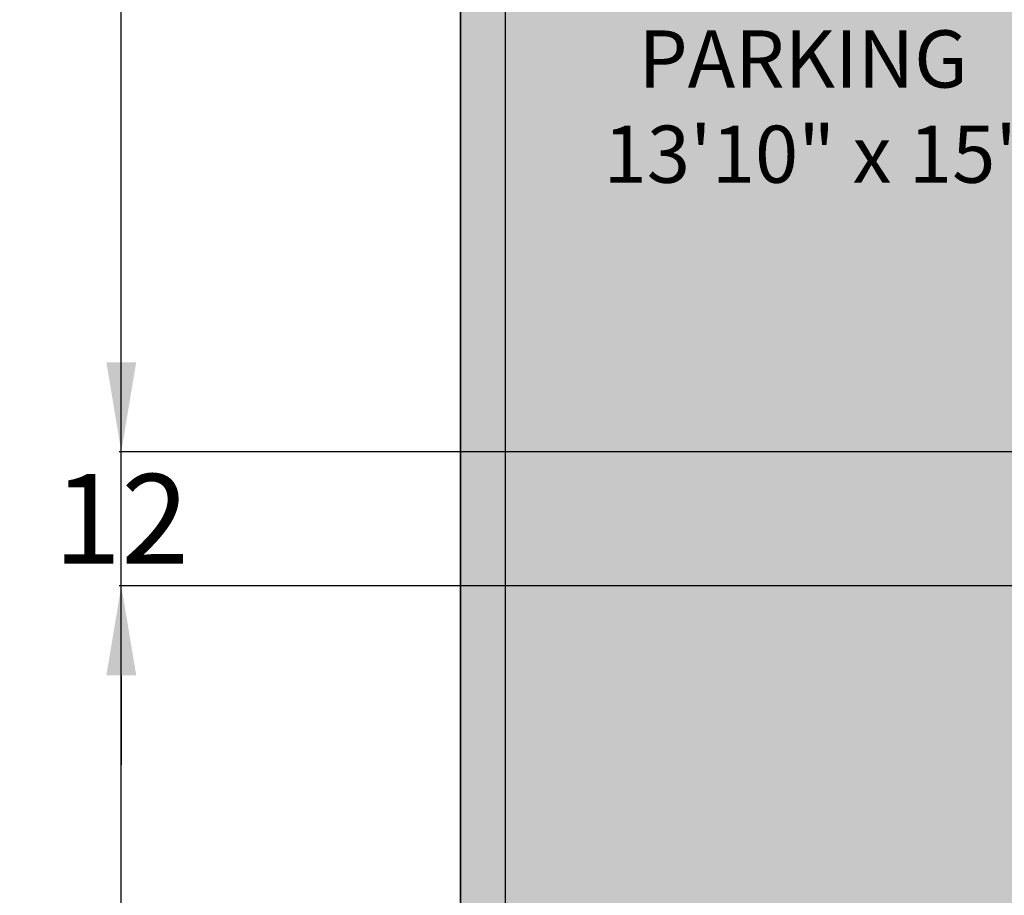
# Model space of a CAD drawing. Units: inches. Extents: x 389 to 971, y 148 to 870.
# Tile 2 of 14: x 389 to 477, y 349 to 428. Entities that reach past the tile are written whole.
import ezdxf

# ---------------------------------------------------------------- set-up
doc = ezdxf.new("R2010")
doc.units = ezdxf.units.IN
doc.header["$MEASUREMENT"] = 0
for name, color, linetype, lineweight in [('A-ANNO-DIMS', 2, 'Continuous', 18), ('A-AREA-IDEN', 7, 'Continuous', 18), ('C-PROP', 7, 'Continuous', 35), ('L-GRND-BASE-PATT', 8, 'Continuous', 13), ('L-WALL', 7, 'Continuous', 30)]:
    doc.layers.add(name, color=color, linetype=linetype, lineweight=lineweight)
doc.layers.add('A-WALL-PATT', color=18, linetype='Continuous', lineweight=13, true_color=0x000000)
doc.layers.add('L-GRND-PATT', color=39, linetype='Continuous', lineweight=13, true_color=0x603913)
doc.styles.get("Standard").update_dxf_attribs({"font": 'arial.ttf'})
doc.dimstyles.get("Standard").update_dxf_attribs({"dimtxt": 8, "dimasz": 8, "dimexe": 0.18, "dimexo": 0.0625, "dimgap": 0.09, "dimtad": 0, "dimtih": 1, "dimtoh": 1, "dimdec": 0, "dimzin": 0, "dimdsep": 46, "dimlunit": 3, "dimtxsty": 'Standard', "dimcen": 0.09, "dimadec": 0, "dimazin": 0, "dimtfac": 1, "dimtdec": 0, "dimtofl": 0, "dimtmove": 0, "dimatfit": 3, "dimfxl": 1, "dimtolj": 1, "dimtzin": 0, "dimarcsym": 0})

# ---------------------------------------------------------------- blocks, each defined once
blk = doc.blocks.new('*D45')
at = {"layer": 'A-ANNO-DIMS', "color": 0, "lineweight": -2, "transparency": 16777216}
for p, q in [((428.1535240000002, 834.6445130000004), (397.7110240000004, 834.6445130000004)), ((397.8910240000004, 826.6445130000004), (397.8910240000005, 538.8190969017736)), ((397.8910240000005, 242.6445130000001), (397.8910240000005, 530.4699290982267)), ((428.1535240000002, 234.6445130000001), (397.7110240000005, 234.6445130000001))]:
    blk.add_line(p, q, dxfattribs=at)
at = {"layer": 'A-ANNO-DIMS', "color": 0, "transparency": 16777216}
for points in [[(396.5576906666671, 826.6445130000004), (399.2243573333337, 826.6445130000004), (397.8910240000004, 834.6445130000004)], [(396.5576906666672, 242.6445130000001), (399.2243573333338, 242.6445130000001), (397.8910240000005, 234.6445130000001)]]:
    blk.add_solid(points, dxfattribs=at)
at = {"layer": 'Defpoints', "color": 0, "transparency": 16777216}
for p in [(397.8910240000004, 834.6445130000004), (428.2160240000002, 834.6445130000004), (428.2160240000002, 234.6445130000001)]:
    blk.add_point(p, dxfattribs=at)
at = {"layer": 'A-ANNO-DIMS', "color": 0, "transparency": 16777216, "insert": (397.8910240000005, 534.6445129999998), "char_height": 8, "attachment_point": 5}
blk.add_mtext('\\A1;600', dxfattribs=at)
blk = doc.blocks.new('*D53')
at = {"layer": 'A-ANNO-DIMS', "color": 0, "lineweight": -2, "transparency": 16777216}
for p, q in [((397.8910240000004, 396.9189020000002), (397.8910240000004, 404.9189020000001)), ((690.1535240000002, 388.9189020000003), (397.7110240000004, 388.9189020000002)), ((690.1535240000002, 376.9189020000001), (397.7110240000005, 376.9189020000001)), ((397.8910240000005, 368.9189020000001), (397.8910240000005, 360.918902))]:
    blk.add_line(p, q, dxfattribs=at)
at = {"layer": 'A-ANNO-DIMS', "color": 0, "transparency": 16777216}
for points in [[(396.5576906666671, 396.9189020000002), (399.2243573333337, 396.9189020000002), (397.8910240000004, 388.9189020000002)], [(396.5576906666671, 368.9189020000001), (399.2243573333338, 368.9189020000001), (397.8910240000005, 376.9189020000001)]]:
    blk.add_solid(points, dxfattribs=at)
at = {"layer": 'Defpoints', "color": 0, "transparency": 16777216}
for p in [(397.8910240000004, 388.9189020000002), (690.2160240000001, 388.9189020000003), (690.2160240000001, 376.9189020000001)]:
    blk.add_point(p, dxfattribs=at)
at = {"layer": 'A-ANNO-DIMS', "color": 0, "transparency": 16777216, "insert": (397.8910240000004, 382.9189019999999), "char_height": 8, "attachment_point": 5}
blk.add_mtext('\\A1;12', dxfattribs=at)

msp = doc.modelspace()

# ---------------------------------------------------------------- hatches: boundary and pattern name
at = {"layer": 'A-WALL-PATT'}
h = msp.add_hatch(color=256, dxfattribs=at)
h.dxf.hatch_style = 1
h.paths.add_polyline_path([(432.2160244416713, 434.6445131961097), (436.3672936601142, 434.6445131961097), (436.3672936601142, 443.6445131961098), (432.2160244416713, 443.6445131961098), (432.2160244416714, 830.6445131961094), (746.2160244416714, 830.6445131961098), (746.2160244416714, 823.8175070811654), (755.2160244416712, 823.8175070811657), (755.2160244416712, 825.6445131961098), (839.2160244416713, 825.6445131961098), (839.2160244416713, 803.5176064986067), (839.2160244416712, 741.6445131961098), (755.2160244416712, 741.6445131961098), (755.2160244416712, 748.4596256139029), (755.1858732057922, 748.4596256139029), (750.7160244416712, 748.4596256139029), (746.2160244416714, 748.4596256139029), (746.2160244416714, 732.6445131961098), (839.2160244416712, 732.6445131961098), (839.2160244416712, 600.6445131961098), (708.5170970640701, 600.6445131961098), (708.5170970640701, 596.1445131961098), (708.5170970640701, 591.6445131961098), (794.2160244416712, 591.6445131961098), (794.2160244416712, 587.4291281246713), (803.2160244416712, 587.4291281246713), (803.2160244416712, 591.6445131961098), (839.2160244416712, 591.6445131961098), (839.2160244416712, 466.6011988194286), (803.2160244416712, 466.6011988194285), (803.2160244416712, 471.0308934694551), (794.2160244416712, 471.0308934694551), (794.2160244416712, 466.6011988194285), (784.6144969105871, 466.6011988194285), (784.6144969105871, 457.6011988194286), (839.2160244416712, 457.6011988194286), (839.2160244416712, 447.6445131961096), (839.2160244416713, 294.6445131961098), (810.0513609197294, 294.6445131961098), (810.0513609197296, 285.6445131961097), (839.2160244416713, 285.6445131961097), (839.2160244416713, 238.6445131961098), (590.2160244416713, 238.6445131961097), (590.2160244416713, 234.6445131961098), (848.2160244416714, 234.6445131961098), (848.2160244416714, 834.6445131961098), (428.2160244416714, 834.6445131961098), (428.2160244416714, 234.6445131961098), (437.2160244416714, 234.6445131961098), (437.2160244416714, 243.6445131961098), (432.2160244416713, 243.6445131961098)])
at = {"layer": 'L-GRND-BASE-PATT'}
h = msp.add_hatch(color=256, dxfattribs=at)
h.dxf.hatch_style = 1
edge = h.paths.add_edge_path(flags=16)
edge.add_ellipse((8782.002602781105, 354.2472542798386), major_axis=(-8296.949265805946, 5.39345e-11), ratio=0.8423038695428886, start_angle=-0.0902290885933894, end_angle=0.3838667787920258, ccw=False)
edge.add_ellipse((485.0533369751568, 368.2895347624687), major_axis=(-1.159084047334488, 1.838e-13), ratio=0.8423038695439892, start_angle=9.094947017729282e-12, end_angle=90.00000000000898, ccw=False)
edge.add_line((483.8942529278224, 368.2895347624687), (483.8942529278225, 387.6039063360424))
edge.add_ellipse((485.0533369751571, 387.2465553762829), major_axis=(1.159084047334488, 1.838e-13), ratio=0.8423038695439892, start_angle=89.99999999999102, end_angle=179.9999999999909, ccw=False)
edge.add_line((485.0533369751572, 388.2228563544795), (485.5047440247956, 388.2228563544795))
edge.add_ellipse((898.8202485054873, 372.489720535918), major_axis=(413.7373561031672, 1.26113e-11), ratio=0.8423038695441164, start_angle=176.3495724142986, end_angle=177.8200496863524, ccw=False)
edge.add_ellipse((535.9119176052733, 196.3854951855018), major_axis=(-245.3971626940985, 1.013648e-10), ratio=0.8423038695442548, start_angle=-77.87403444769302, end_angle=-76.2194710104792, ccw=False)
edge.add_ellipse((535.9119176052684, 201.7546502845751), major_axis=(239.1273775699096, 1.008988e-10), ratio=0.842303869543627, start_angle=100.20953899711827, end_angle=102.44462729341922, ccw=False)
edge.add_ellipse((473.3138688667988, 564.9222417143382), major_axis=(196.5636751472093, 8.4793e-12), ratio=0.8423038695439335, start_angle=-80.74343399280163, end_angle=-77.44506735586587)
edge.add_line((509.5535496243029, 402.1940957519602), (514.3535105156315, 404.8483349684994))
edge.add_line((514.3535105156315, 404.8483349684994), (514.3535105156315, 404.7971763262221))
edge.add_ellipse((514.3535105156316, 404.2643898676136), major_axis=(0.5795420236673633, 2e-16), ratio=0.8423038695437671, start_angle=52.06686954015339, end_angle=90.00000000001342, ccw=False)
edge.add_line((514.671564037824, 404.672460591463), (519.1534714069603, 402.19409575196))
edge.add_ellipse((555.3931521644682, 564.9222417143374), major_axis=(-196.5636751472384, 3.62381e-11), ratio=0.8423038695438114, start_angle=77.44506735587258, end_angle=80.74343399280833)
edge.add_ellipse((492.795103425985, 201.7546502845724), major_axis=(239.12737756976, 4.82267e-11), ratio=0.8423038695441539, start_angle=77.55537270654253, end_angle=79.7904610028433, ccw=False)
edge.add_ellipse((492.7951034259847, 196.3854951855023), major_axis=(245.3971626940514, 1.422861e-10), ratio=0.8423038695444116, start_angle=76.21947101046823, end_angle=77.87403444768199, ccw=False)
edge.add_ellipse((129.8867725257751, 372.4897205359271), major_axis=(-413.7373561031673, 2.44623e-11), ratio=0.8423038695441432, start_angle=182.179950313648, end_angle=183.6504275857018, ccw=False)
edge.add_line((543.2022770064673, 388.2228563544788), (544.0779382625514, 388.2228563544787))
edge.add_ellipse((543.6536840561057, 387.2465553762822), major_axis=(-1.159084047334545, 1.527e-13), ratio=0.8423038695438989, start_angle=180.0000000000075, end_angle=270.00000000000756, ccw=False)
edge.add_line((544.8127681034401, 387.2465553762826), (544.8127681034399, 367.9321838027083))
edge.add_ellipse((543.6536840561054, 368.2895347624679), major_axis=(1.159084047334544, 7.24e-14), ratio=0.8423038695439478, start_angle=269.9999999999964, end_angle=359.9999999999964, ccw=False)
edge.add_ellipse((-7753.295581726658, 354.2472542799028), major_axis=(-8296.949265782761, 2.068448e-10), ratio=0.8423038695442414, start_angle=179.6161332212083, end_angle=180.0902290885951, ccw=False)
edge.add_line((543.3912265319653, 298.6607849184036), (544.0779382625504, 298.6607849184036))
edge.add_ellipse((543.6536840561046, 297.6844839402071), major_axis=(1.159084047334431, 1.769e-13), ratio=0.8423038695439814, start_angle=-1.1482370609883219e-11, end_angle=89.99999999999119, ccw=False)
edge.add_line((544.8127681034391, 297.684483940207), (544.8127681034387, 278.3701123666333))
edge.add_ellipse((543.6536840561043, 278.727463326393), major_axis=(-1.159084047334431, 2.574e-13), ratio=0.8423038695440306, start_angle=90.00000000001268, end_angle=180.0000000000099, ccw=False)
edge.add_line((543.6536840561045, 277.7511623481965), (543.1566278692261, 277.7511623481965))
edge.add_ellipse((-7753.295581726658, 354.2472542799028), major_axis=(-8296.949265782761, 2.068448e-10), ratio=0.8423038695442414, start_angle=179.3813568036816, end_angle=179.4717285281829, ccw=False)
edge.add_ellipse((542.4236240941387, 263.2762864208561), major_axis=(-1.738626071001761, 2.132e-13), ratio=0.8423038695439151, start_angle=179.3717627838137, end_angle=248.464756601011, ccw=False)
edge.add_ellipse((-7753.875123750511, 354.2472542780016), major_axis=(-8298.740341433751, 2.4782644722e-06), ratio=0.8423038662721074, start_angle=179.3534459200609, end_angle=179.3717628008941, ccw=False)
edge.add_ellipse((540.0116322079951, 260.6509346628677), major_axis=(-4.109243751168186, 2.384e-13), ratio=0.842303869543976, start_angle=90.0000000000635, end_angle=179.3534459029233, ccw=False)
edge.add_line((540.0116322079991, 257.1897027503593), (488.6953888232593, 257.1897027503609))
edge.add_ellipse((488.6953888232669, 260.6509346628715), major_axis=(4.10924375117072, 1.262e-13), ratio=0.8423038695439824, start_angle=180.6465540970565, end_angle=269.9999999998589, ccw=False)
edge.add_ellipse((8782.582144816053, 354.2472542821698), major_axis=(-8298.740341477976, 1.8591886369e-06), ratio=0.8423038720186145, start_angle=0.6282372290784792, end_angle=0.6465541099116194, ccw=False)
edge.add_ellipse((486.2833969371199, 263.2762864208594), major_axis=(-1.738626071002378, 2.7e-13), ratio=0.8423038695439394, start_angle=-68.46475649596817, end_angle=0.6282372161796275, ccw=False)
edge.add_ellipse((8782.002602781105, 354.2472542798386), major_axis=(-8296.949265805946, 5.39345e-11), ratio=0.8423038695428886, start_angle=0.5282714718171064, end_angle=0.6465540970606867, ccw=False)
edge.add_line((485.5503931620382, 277.7511623481972), (484.6290827687102, 277.7511623481972))
edge.add_ellipse((485.0533369751559, 278.7274633263938), major_axis=(-1.159084047334545, 3.11e-13), ratio=0.8423038695439968, start_angle=1.5404566511278972e-11, end_angle=90.000000000012, ccw=False)
edge.add_line((483.8942529278214, 278.7274633263938), (483.8942529278216, 298.0418348999672))
edge.add_ellipse((485.053336975156, 297.6844839402078), major_axis=(1.159084047334488, 1.025e-13), ratio=0.8423038695440382, start_angle=89.99999999999488, end_angle=179.9999999999949, ccw=False)
edge = h.paths.add_edge_path(flags=0)
edge.add_ellipse((8782.002602781096, 354.247254279773), major_axis=(-8295.790181758603, 9.87839e-10), ratio=0.8423038695486498, start_angle=0.05559431350519617, end_angle=0.37776419391582294, ccw=False)
edge.add_line((486.2179253655185, 346.1978202249628), (489.3905023836935, 335.8383575186984))
edge.add_ellipse((3386.011413077446, 329.726312794031), major_axis=(-2896.629999631248, 1.069454e-10), ratio=0.8423038695494893, start_angle=-0.1208973690315206, end_angle=0.3640763488915184)
edge.add_line((489.4638383140943, 311.3204429697198), (486.4665645878948, 299.5520931219791))
edge = h.paths.add_edge_path(flags=0)
edge.add_ellipse((514.3535105156315, 391.3730654902235), major_axis=(-115.1512533244504, 1.8736e-12), ratio=0.8423038695439684, start_angle=76.4018653097696, end_angle=103.5981346902308)
edge.add_line((537.3427693057832, 296.3333211885938), (537.342769305783, 281.5897392316151))
edge.add_ellipse((514.3535105156313, 376.6294835332447), major_axis=(-115.1512533244486, 9.02e-13), ratio=0.8423038695439828, start_angle=76.40186530976922, end_angle=103.59813469023032, ccw=False)
edge.add_line((491.3642517254773, 281.5897392316156), (491.3642517254774, 296.3333211885945))
edge = h.paths.add_edge_path(flags=0)
edge.add_line((491.3642517254777, 337.0752369161334), (489.6529508739416, 349.9015767089268))
edge.add_ellipse((510.1338164488795, 298.7862183048575), major_axis=(64.04807894948699, 3.9006e-12), ratio=0.8423038695439252, start_angle=94.27742096304979, end_angle=111.83495379670401, ccw=False)
edge.add_line((506.106812905481, 352.6274231954524), (522.600208125781, 352.6274231954521))
edge.add_ellipse((518.5732045823798, 298.7862183048586), major_axis=(64.04807894948067, 3.24e-14), ratio=0.8423038695439885, start_angle=68.16504620328948, end_angle=85.72257903694378, ccw=False)
edge.add_line((539.05407015732, 349.9015767089259), (537.3427693057835, 337.0752369161327))
edge.add_ellipse((516.5461636849332, 287.5825181681899), major_axis=(62.33048198262021, 1.5954e-12), ratio=0.8423038695439995, start_angle=67.20808512240782, end_angle=85.12993040286212)
edge.add_line((521.0080028322477, 339.9490379899644), (507.6990181990146, 339.9490379899646))
edge.add_ellipse((512.1608573463288, 287.5825181681774), major_axis=(62.33048198263887, 2.0798e-12), ratio=0.8423038695439498, start_angle=94.8700695971331, end_angle=112.791914877584)
edge = h.paths.add_edge_path(flags=0)
edge.add_ellipse((493.6824198201462, 273.9438556676354), major_axis=(-2.318168094668919, 1.896e-13), ratio=0.8423038695439611, start_angle=-89.99999999999523, end_angle=4.718003765447065e-12, ccw=False)
edge.add_line((493.6824198201462, 275.8964576240284), (535.3743409680425, 275.8964576240277))
edge.add_ellipse((535.024601211114, 273.9438556676347), major_axis=(2.318168094668976, 2.946e-13), ratio=0.8423038695439647, start_angle=-7.275957614183426e-12, end_angle=89.99999999998943, ccw=False)
edge.add_line((537.342769305783, 273.9438556676347), (537.3427693057827, 258.698332706474))
edge.add_line((537.3427693057827, 258.698332706474), (540.5911742316662, 258.6983327064739))
edge.add_ellipse((540.5911742316634, 260.6509346628669), major_axis=(-2.318168094668839, 2.143e-13), ratio=0.8423038695440144, start_angle=90.00000000008203, end_angle=179.3534459029346)
edge.add_line((540.5911742316662, 258.6983327064739), (487.7691399811528, 258.6983327064755))
edge.add_ellipse((488.1158467995968, 260.6509346628684), major_axis=(2.318168094668909, 7.48e-14), ratio=0.8423038695439647, start_angle=180.6465540970884, end_angle=269.9999999999081)
edge.add_line((488.1158467995931, 258.6983327064755), (491.3642517254771, 258.6983327064754))
edge.add_line((491.3642517254771, 258.6983327064754), (491.3642517254771, 274.2384428182294))
h.paths.add_polyline_path([(746.1375687288224, 327.3223047166553), (750.1400147212453, 327.3223047166553), (750.1400147212453, 326.2830696147227), (798.1693712998389, 326.2830696147227), (798.1693712998389, 327.3223047166553), (802.1718172922616, 327.3223047166553), (802.1718172922616, 309.9783792024682, -0.1904762075443491), (746.1375687288224, 309.9783668090107)], flags=16)
h.paths.add_polyline_path([(782.1595875801748, 313.5684994305933), (782.1595893317732, 309.0414930416419, -0.0496282101666581), (766.1497986905329, 309.0414910503953), (766.1498004421323, 313.5684994305933)], flags=0)
h.paths.add_polyline_path([(755.1858908233534, 344.9352232902417), (755.1858908233534, 373.916311072083), (788.1243995226009, 373.916311072083), (788.1243995226009, 344.9352232902417)], flags=16)
h.paths.add_polyline_path([(757.1858908233535, 346.9352232902417), (757.1858908233535, 371.916311072083), (786.1243995226009, 371.916311072083), (786.1243995226009, 346.9352232902417)], flags=0)
h.paths.add_polyline_path([(803.6445810111745, 338.4878931208803), (803.6445810111745, 342.4903391133031), (804.6838161131072, 342.4903391133031), (804.6838161131072, 390.5196956918968), (803.6445810111748, 390.5196956918968), (803.6445810111748, 394.5221416843196), (820.9885065253617, 394.5221416843196, -0.1904762075443491), (820.9885189188192, 338.4878931208803)], flags=16)
h.paths.add_polyline_path([(806.8706930931005, 326.6963103558256), (806.4254411777042, 327.1415622712219), (806.4723791864895, 326.6297175483474)], flags=16)
h.paths.add_polyline_path([(822.0328146004263, 317.4007976138144), (822.1941503181826, 317.8932883068639), (821.562628166435, 317.9885306563034)], flags=16)
h.paths.add_polyline_path([(817.3983862972365, 358.5001248341902), (817.3983862972365, 374.5099119722327), (821.9253926861879, 374.5099137238312, -0.049628210166658), (821.9253946774346, 358.5001230825909)], flags=0)
h.paths.add_polyline_path([(808.1446344648577, 418.9736619306146), (808.2246858861593, 418.5632188717996), (808.5395491501399, 418.5787472453325)], flags=16)
h.paths.add_polyline_path([(820.3158762739024, 412.6690288868844), (820.4772119916585, 413.161519579934), (819.8456898399113, 413.2567619293735)], flags=16)
h.paths.add_polyline_path([(466.3155093563569, 235.5246322146605), (517.3806533266912, 235.5246322146605), (517.3806533266912, 244.4269231682286), (466.3155093563569, 244.4269231682286)], flags=24)
h.paths.add_polyline_path([(739.8737195480014, 256.2000079819968), (815.4040239338423, 256.2000079819968), (815.4040239338423, 265.3453807094367), (739.8737195480014, 265.3453807094367)], flags=24)
h.paths.add_polyline_path([(750.6081538187397, 393.6666679930368), (791.5680640722773, 393.6666679930368), (791.5680640722773, 412.3933175868746), (750.6081538187397, 412.3933175868746)], flags=24)
h.paths.add_polyline_path([(438.9630812812552, 410.0618566955462), (484.6203810968238, 410.0618566955462), (484.6203810968238, 429.1217352891893), (438.9630812812552, 429.1217352891893)], flags=24)
edge = h.paths.add_edge_path()
edge.add_line((839.2160244416713, 285.6445131961097), (611.8786784019748, 285.6445131961099))
edge.add_line((611.8786784019748, 285.6445131961099), (604.3870116090119, 285.6445131961097))
edge.add_line((604.3870116090119, 285.6445131961097), (595.3870116090119, 285.6445131961097))
edge.add_line((595.3870116090119, 285.6445131961097), (595.3870116090118, 370.1553848722774))
edge.add_line((595.3870116090118, 370.1553848722774), (604.0816928471932, 370.1553848722774))
edge.add_line((604.0816928471932, 370.1553848722774), (604.0816928471932, 371.3788335667469))
edge.add_line((604.0816928471932, 371.3788335667469), (632.0194586761203, 371.3788335667469))
edge.add_arc((604.0816928471932, 370.1553848722773), 27.96454158787471, 2.507490703587644, 90.00000000000003)
edge.add_line((604.0816928471932, 398.1199264601519), (599.8870116090108, 398.1652144688576))
edge.add_line((599.8870116090108, 398.1652144688576), (604.4225424425357, 398.1652144688576))
edge.add_arc((604.4225424425357, 428.4020866923496), 30.23687222349201, 270.0000000000002, 357.492509296413)
edge.add_line((634.6304631740308, 427.0792235325719), (604.4225424425357, 427.0792235325719))
edge.add_line((604.4225424425357, 427.0792235325719), (604.4225424425357, 428.4020866923497))
edge.add_line((604.4225424425357, 428.4020866923497), (599.8870116090119, 428.4020866923497))
edge.add_line((599.8870116090119, 428.4020866923497), (595.3870116090116, 428.4020866923497))
edge.add_line((595.3870116090116, 428.4020866923497), (595.3870116090118, 434.6445131961097))
edge.add_line((595.3870116090118, 434.6445131961097), (585.0790669792458, 434.6445131961097))
edge.add_line((585.0790669792458, 434.6445131961097), (540.3921730610418, 434.6445131961097))
edge.add_line((540.3921730610418, 434.6445131961097), (526.712508448134, 434.6445131961097))
edge.add_line((526.712508448134, 434.6445131961097), (488.4094553949635, 434.6445131961097))
edge.add_line((488.4094553949635, 434.6445131961097), (432.2160244416713, 434.6445131961097))
edge.add_line((432.2160244416713, 434.6445131961097), (432.2160244416713, 243.6445131961098))
edge.add_line((432.2160244416713, 243.6445131961098), (437.2160244416714, 243.6445131961098))
edge.add_line((437.2160244416714, 243.6445131961098), (437.2160244416714, 234.6445131961098))
edge.add_line((437.2160244416714, 234.6445131961098), (581.2160244416713, 234.6445131961098))
edge.add_line((581.2160244416713, 234.6445131961098), (581.2160244416713, 238.6445131961097))
edge.add_line((581.2160244416713, 238.6445131961097), (581.2160244416713, 243.6445131961098))
edge.add_line((581.2160244416713, 243.6445131961098), (590.2160244416713, 243.6445131961098))
edge.add_line((590.2160244416713, 243.6445131961098), (590.2160244416713, 238.6445131961097))
edge.add_line((590.2160244416713, 238.6445131961097), (839.2160244416713, 238.6445131961098))
edge.add_line((839.2160244416713, 238.6445131961098), (839.2160244416713, 285.6445131961097))
at = {"layer": 'L-GRND-PATT'}
h = msp.add_hatch(dxfattribs=at)
h.set_pattern_fill('EARTH', color=256, angle=45)
h.set_pattern_definition([(45, (0, 0), (0, 8.980256121069154), [6.349999999999999, -6.349999999999999]), (45, (-1.683798022700466, 1.683798022700466), (0, 8.980256121069154), [6.349999999999999, -6.349999999999999]), (45, (-3.367596045400933, 3.367596045400933), (0, 8.980256121069154), [6.349999999999999, -6.349999999999999]), (135, (-3.367596045400933, 4.490128060534576), (-8.980256121069154, 0), [6.349999999999999, -6.349999999999999]), (135, (-1.683798022700466, 6.173926083235043), (-8.980256121069154, 0), [6.349999999999999, -6.349999999999999]), (135, (0, 7.85772410593551), (-8.980256121069154, 0), [6.349999999999999, -6.349999999999999])])
h.paths.add_polyline_path([(432.2160244416713, 243.6445131961098), (437.2160244416714, 243.6445131961098), (437.2160244416714, 234.6445131961098), (581.2160244416713, 234.6445131961098), (581.2160244416713, 238.6445131961097), (581.2160244416713, 243.6445131961098), (590.2160244416713, 243.6445131961098), (590.2160244416713, 238.6445131961097), (839.2160244416713, 238.6445131961098), (839.2160244416712, 285.6445131961097), (810.0513609197296, 285.6445131961097), (733.8056934525983, 285.6445131961099), (684.2433676403508, 285.6445131961098), (611.8786784019748, 285.6445131961099), (604.3870116090119, 285.6445131961097), (595.3870116090119, 285.6445131961097), (595.3870116090118, 370.1553848722774), (604.0816928471932, 370.1553848722774), (604.0816928471932, 371.3788335667469), (632.0194586761203, 371.3788335667469, 0.4014527144963568), (604.0816928471932, 398.119926460152), (599.8870116090127, 398.1652144688576), (604.4225424425357, 398.1652144688576, 0.4014527144963579), (634.6304631740308, 427.0792235325719), (604.4225424425357, 427.0792235325719), (604.4225424425357, 428.4020866923497), (599.8870116090119, 428.4020866923497), (595.3870116090116, 428.4020866923497), (595.3870116090118, 434.6445131961097), (585.0790669792458, 434.6445131961097), (540.3921730610418, 434.6445131961097), (526.712508448134, 434.6445131961097), (488.4094553949635, 434.6445131961097), (432.2160244416713, 434.6445131961097)])
edge = h.paths.add_edge_path(flags=16)
edge.add_line((483.8942529278214, 278.7274633263938), (483.8942529278216, 298.2563878122772))
edge.add_ellipse((485.053336975156, 297.6844839402078), major_axis=(1.159084047334488, 1.025e-13), ratio=0.8423038695440382, start_angle=89.99999999999488, end_angle=179.9999999999949, ccw=False)
edge.add_ellipse((8782.002602781105, 354.2472542798386), major_axis=(-8296.949265805946, 5.39345e-11), ratio=0.8423038695428886, start_angle=-0.0902290885933894, end_angle=0.3838667787920258, ccw=False)
edge.add_ellipse((485.0533369751568, 368.2895347624687), major_axis=(-1.159084047334488, 1.838e-13), ratio=0.8423038695439892, start_angle=9.094947017729282e-12, end_angle=90.00000000000898, ccw=False)
edge.add_line((483.8942529278224, 368.2895347624687), (483.8942529278225, 387.8184592483523))
edge.add_ellipse((485.0533369751571, 387.2465553762829), major_axis=(1.159084047334488, 1.838e-13), ratio=0.8423038695439892, start_angle=89.99999999999102, end_angle=179.9999999999909, ccw=False)
edge.add_ellipse((898.8202485054873, 372.489720535918), major_axis=(413.7373561031672, 1.26113e-11), ratio=0.8423038695441164, start_angle=176.3495724142986, end_angle=177.8200496863524, ccw=False)
edge.add_ellipse((535.9119176052733, 196.3854951855018), major_axis=(-245.3971626940985, 1.013648e-10), ratio=0.8423038695442548, start_angle=-77.87403444769302, end_angle=-76.2194710104792, ccw=False)
edge.add_ellipse((535.9119176052684, 201.7546502845751), major_axis=(239.1273775699096, 1.008988e-10), ratio=0.842303869543627, start_angle=100.20953899711827, end_angle=102.44462729341922, ccw=False)
edge.add_ellipse((473.3138688667988, 564.9222417143382), major_axis=(196.5636751472093, 8.4793e-12), ratio=0.8423038695439335, start_angle=-80.74343399280163, end_angle=-77.44506735586587)
edge.add_line((509.5535496243029, 402.1940957519602), (514.3535105156316, 404.8483349684994))
edge.add_line((514.3535105156316, 404.8483349684994), (519.1534714069603, 402.19409575196))
edge.add_ellipse((555.3931521644682, 564.9222417143374), major_axis=(-196.5636751472384, 3.62381e-11), ratio=0.8423038695438114, start_angle=77.44506735587258, end_angle=80.74343399280833)
edge.add_ellipse((492.795103425985, 201.7546502845724), major_axis=(239.12737756976, 4.82267e-11), ratio=0.8423038695441539, start_angle=77.55537270654253, end_angle=79.7904610028433, ccw=False)
edge.add_ellipse((492.7951034259847, 196.3854951855023), major_axis=(245.3971626940514, 1.422861e-10), ratio=0.8423038695444116, start_angle=76.21947101046823, end_angle=77.87403444768199, ccw=False)
edge.add_ellipse((129.8867725257751, 372.4897205359271), major_axis=(-413.7373561031673, 2.44623e-11), ratio=0.8423038695441432, start_angle=182.179950313648, end_angle=183.6504275857018, ccw=False)
edge.add_line((543.2022770064673, 388.2228563544789), (544.3326597711041, 388.2228563544786))
edge.add_ellipse((543.6536840561057, 387.2465553762822), major_axis=(-1.159084047334545, 1.527e-13), ratio=0.8423038695438989, start_angle=180.0000000000075, end_angle=270.00000000000756, ccw=False)
edge.add_line((544.8127681034401, 387.2465553762825), (544.8127681034399, 367.7176308903986))
edge.add_ellipse((543.6536840561054, 368.2895347624679), major_axis=(1.159084047334544, 7.24e-14), ratio=0.8423038695439478, start_angle=269.9999999999964, end_angle=359.9999999999964, ccw=False)
edge.add_ellipse((-7753.295581726658, 354.2472542799028), major_axis=(-8296.949265782761, 2.068448e-10), ratio=0.8423038695442414, start_angle=179.6161332212083, end_angle=180.0902290885951, ccw=False)
edge.add_ellipse((543.6536840561046, 297.6844839402071), major_axis=(1.159084047334431, 1.769e-13), ratio=0.8423038695439814, start_angle=-1.1482370609883219e-11, end_angle=89.99999999999119, ccw=False)
edge.add_line((544.8127681034391, 297.6844839402071), (544.8127681034387, 278.1555594543235))
edge.add_ellipse((543.6536840561043, 278.727463326393), major_axis=(-1.159084047334431, 2.574e-13), ratio=0.8423038695440306, start_angle=90.00000000001268, end_angle=180.0000000000099, ccw=False)
edge.add_ellipse((-7753.295581726658, 354.2472542799028), major_axis=(-8296.949265782761, 2.068448e-10), ratio=0.8423038695442414, start_angle=179.3813568036816, end_angle=179.4717285281829, ccw=False)
edge.add_ellipse((542.4236240941387, 263.2762864208561), major_axis=(-1.738626071001761, 2.132e-13), ratio=0.8423038695439151, start_angle=179.3717627838137, end_angle=248.464756601011, ccw=False)
edge.add_ellipse((-7753.875123750511, 354.2472542780016), major_axis=(-8298.740341433751, 2.4782644722e-06), ratio=0.8423038662721074, start_angle=179.3534459200609, end_angle=179.3717628008941, ccw=False)
edge.add_ellipse((540.0116322079951, 260.6509346628677), major_axis=(-4.109243751168186, 2.384e-13), ratio=0.842303869543976, start_angle=90.0000000000635, end_angle=179.3534459029233, ccw=False)
edge.add_line((540.0116322079989, 257.1897027503593), (488.0808074948215, 257.1897027503609))
edge.add_ellipse((488.6953888232669, 260.6509346628715), major_axis=(4.10924375117072, 1.262e-13), ratio=0.8423038695439824, start_angle=180.6465540970565, end_angle=269.9999999998589, ccw=False)
edge.add_ellipse((8782.582144816053, 354.2472542821698), major_axis=(-8298.740341477976, 1.8591886369e-06), ratio=0.8423038720186145, start_angle=0.6282372290784792, end_angle=0.6465541099116194, ccw=False)
edge.add_ellipse((486.2833969371199, 263.2762864208594), major_axis=(-1.738626071002378, 2.7e-13), ratio=0.8423038695439394, start_angle=-68.46475649596817, end_angle=0.6282372161796275, ccw=False)
edge.add_ellipse((8782.002602781105, 354.2472542798386), major_axis=(-8296.949265805946, 5.39345e-11), ratio=0.8423038695428886, start_angle=0.5282714718171064, end_angle=0.6465540970606867, ccw=False)
edge.add_line((485.5503931620382, 277.7511623481972), (484.3743612601578, 277.7511623481972))
edge.add_ellipse((485.0533369751559, 278.7274633263938), major_axis=(-1.159084047334545, 3.11e-13), ratio=0.8423038695439968, start_angle=1.5404566511278972e-11, end_angle=90.000000000012, ccw=False)
edge = h.paths.add_edge_path(flags=0)
edge.add_ellipse((488.1158467995968, 260.6509346628684), major_axis=(2.318168094668909, 7.48e-14), ratio=0.8423038695439647, start_angle=180.6465540970884, end_angle=269.9999999999081)
edge.add_line((488.1158467995933, 258.6983327064755), (491.3642517254771, 258.6983327064753))
edge.add_line((491.3642517254771, 258.6983327064753), (491.3642517254771, 274.4686391213292))
edge.add_ellipse((493.6824198201462, 273.9438556676354), major_axis=(-2.318168094668919, 1.896e-13), ratio=0.8423038695439611, start_angle=-89.99999999999523, end_angle=4.718003765447065e-12, ccw=False)
edge.add_line((493.6824198201462, 275.8964576240284), (535.6476346230087, 275.8964576240277))
edge.add_ellipse((535.024601211114, 273.9438556676347), major_axis=(2.318168094668976, 2.946e-13), ratio=0.8423038695439647, start_angle=-7.275957614183426e-12, end_angle=89.99999999998943, ccw=False)
edge.add_line((537.342769305783, 273.9438556676347), (537.3427693057827, 258.698332706474))
edge.add_line((537.3427693057827, 258.698332706474), (541.2086129152347, 258.6983327064739))
edge.add_ellipse((540.5911742316634, 260.6509346628669), major_axis=(-2.318168094668839, 2.143e-13), ratio=0.8423038695440144, start_angle=90.00000000008203, end_angle=179.3534459029347, ccw=False)
edge.add_line((540.5911742316662, 258.6983327064739), (487.4984081160257, 258.6983327064755))
edge = h.paths.add_edge_path(flags=0)
edge.add_line((491.3642517254773, 281.5897392316156), (491.3642517254774, 296.3333211885945))
edge.add_ellipse((514.3535105156315, 391.3730654902235), major_axis=(-115.1512533244504, 1.8736e-12), ratio=0.8423038695439684, start_angle=76.4018653097696, end_angle=103.5981346902308)
edge.add_line((537.3427693057832, 296.3333211885938), (537.342769305783, 281.5897392316151))
edge.add_ellipse((514.3535105156313, 376.6294835332447), major_axis=(-115.1512533244486, 9.02e-13), ratio=0.8423038695439828, start_angle=76.40186530976922, end_angle=103.59813469023032, ccw=False)
edge = h.paths.add_edge_path(flags=0)
edge.add_ellipse((8782.002602781096, 354.247254279773), major_axis=(-8295.790181758603, 9.87839e-10), ratio=0.8423038695486498, start_angle=0.05559431350519617, end_angle=0.37776419391582294, ccw=False)
edge.add_line((486.2179253655185, 346.1978202249628), (489.3905023836935, 335.8383575186985))
edge.add_ellipse((3386.011413077446, 329.726312794031), major_axis=(-2896.629999631248, 1.069454e-10), ratio=0.8423038695494893, start_angle=-0.1208973690315206, end_angle=0.3640763488915184)
edge.add_line((489.4638383140943, 311.3204429697198), (486.4665645878948, 299.5520931219782))
edge = h.paths.add_edge_path(flags=0)
edge.add_line((491.3642517254777, 337.0752369161334), (489.6529508739416, 349.9015767089268))
edge.add_ellipse((510.1338164488795, 298.7862183048575), major_axis=(64.04807894948699, 3.9006e-12), ratio=0.8423038695439252, start_angle=94.27742096304979, end_angle=111.83495379670401, ccw=False)
edge.add_line((506.106812905481, 352.6274231954524), (522.600208125781, 352.6274231954521))
edge.add_ellipse((518.5732045823798, 298.7862183048586), major_axis=(64.04807894948067, 3.24e-14), ratio=0.8423038695439885, start_angle=68.16504620328948, end_angle=85.72257903694378, ccw=False)
edge.add_line((539.05407015732, 349.9015767089259), (537.3427693057835, 337.0752369161327))
edge.add_ellipse((516.5461636849332, 287.5825181681899), major_axis=(62.33048198262021, 1.5954e-12), ratio=0.8423038695439995, start_angle=67.20808512240782, end_angle=85.12993040286212)
edge.add_line((521.0080028322477, 339.9490379899644), (507.6990181990145, 339.9490379899646))
edge.add_ellipse((512.1608573463288, 287.5825181681774), major_axis=(62.33048198263887, 2.0798e-12), ratio=0.8423038695439498, start_angle=94.8700695971331, end_angle=112.791914877584)
h.paths.add_polyline_path([(466.3155093563569, 235.5246322146605), (517.3806533266912, 235.5246322146605), (517.3806533266912, 244.4269231682286), (466.3155093563569, 244.4269231682286)], flags=24)
h.paths.add_polyline_path([(739.8737195480014, 256.2000079819968), (815.4040239338423, 256.2000079819968), (815.4040239338423, 265.3453807094367), (739.8737195480014, 265.3453807094367)], flags=24)
h.paths.add_polyline_path([(438.9630812812552, 410.0618566955462), (484.6203810968238, 410.0618566955462), (484.6203810968238, 429.1217352891893), (438.9630812812552, 429.1217352891893)], flags=24)

# ---------------------------------------------------------------- linework, layer by layer
at = {"layer": 'C-PROP'}
msp.add_line((428.2160244416714, 834.6445131961098), (428.2160244416714, 234.6445131961096), dxfattribs=at)
at = {"layer": 'L-WALL'}
msp.add_line((432.2160244416713, 434.6445131961097), (432.2160244416713, 294.6445131961098), dxfattribs=at)

# ---------------------------------------------------------------- texts
at = {"layer": 'A-AREA-IDEN', "insert": (441.017032612244, 426.5799922935042), "char_height": 5.107875574604968, "attachment_point": 1}
msp.add_mtext_dynamic_manual_height_columns('  PARKING\\P13\'10" x 15\'3"', width=115.9269957180866, gutter_width=25.53937787302484, heights=[0], dxfattribs=at)

# ---------------------------------------------------------------- dimensions: what is measured, and where the dimension line sits
at = {"layer": 'A-ANNO-DIMS'}
for base, p1, p2, picture, middle in [((397.8910240000004, 834.6445130000004), (428.216024, 234.644513), (428.216024, 834.6445129999998), '*D45', (397.8910240000005, 534.6445129999998)), ((397.8910240000004, 388.9189020000002), (690.216024, 376.918902), (690.216024, 388.918902), '*D53', (397.8910240000004, 382.9189019999999))]:
    dim = msp.add_linear_dim(base=base, p1=p1, p2=p2, angle=90, dimstyle='Standard', override={"dimdec": 0, "dimlfac": 1, "dimrnd": 0, "dimzin": 0, "dimdsep": 46, "dimlunit": 2}, dxfattribs=at)
    dim.commit()
    dim.dimension.update_dxf_attribs({"geometry": picture, "text_midpoint": middle})

doc.saveas('drawing.dxf')
